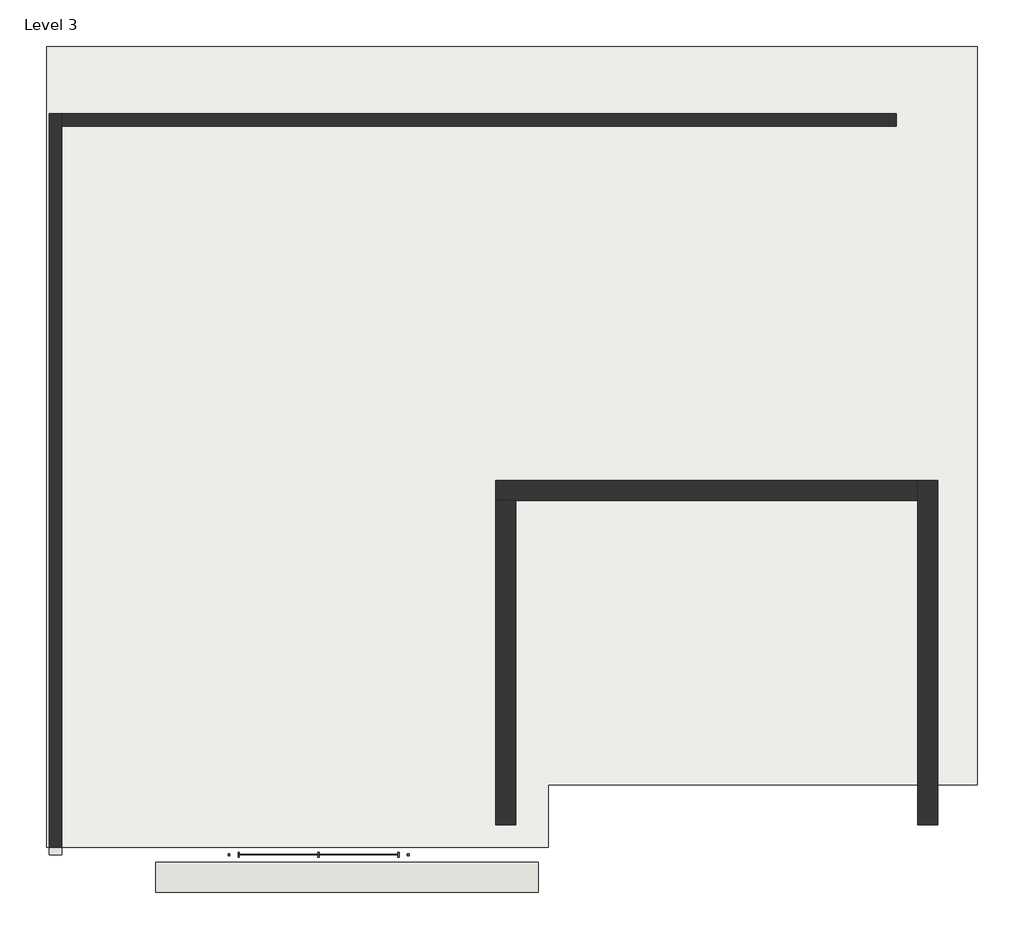
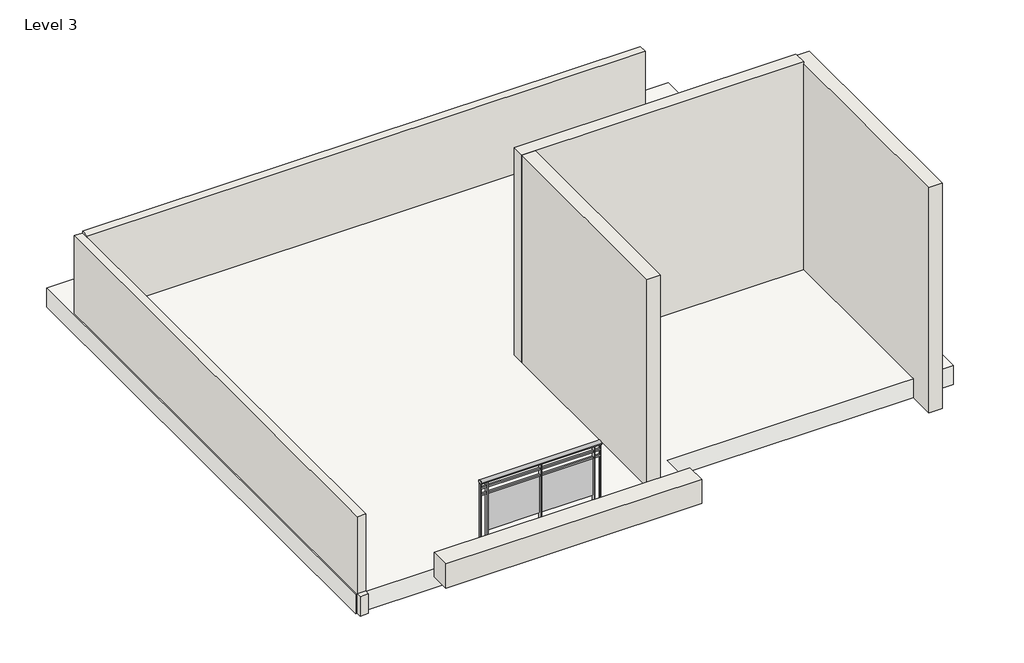
# One storey: 6 walls, 1 railing, 1 roof.
"""IFC4 building model written with IfcOpenShell, lengths in millimetres."""

from ifc_helpers import new_model, si_unit, point, frame, origin, place, context, project, spatial, polyline, ellipse_curve, trimmed, outline, extrude, faceted_brep, transform, mapped, element, save
from ifc_brep_helpers import plane_surface, extruded_surface, advanced_brep
from components import walls_3_walls_3_34f02fba

model = new_model("IFC4")

# Units and contexts
model_context = context("Model", 3, world=origin())
ifc_project = project(units=[si_unit("LENGTHUNIT", "METRE", prefix="MILLI")], contexts=[model_context])

# Site, building, storey
site = spatial("IfcSite", under=ifc_project)
building = spatial("IfcBuilding", under=site)
storey = spatial("IfcBuildingStorey", under=building, Name="Level 3", Elevation=7315.2)

# Railing
placement = place(None, origin())
element("IfcRailing", 1, ObjectType="Glass Panel - Bottom Fill", at=placement, inside=storey, context=model_context, shape_type="SolidModel", body=[
    advanced_brep(
    [(-8387.3093643, 1747.2827135, 8839.2), (-8387.3093643, 1671.0827135, 8839.2), (-6558.5093643, 1747.2827135, 8839.2), (-6558.5093643, 1671.0827135, 8839.2)],
    [
        (0, 1, ellipse_curve(frame((-8387.3093643, 1709.1827135, 8839.2), z_axis=(-1.0, 0.0, 0.0), x_axis=(0.0, -1.0, 0.0)), 38.1, 28.575)),
        (1, 0, ellipse_curve(frame((-8387.3093643, 1709.1827135, 8839.2), z_axis=(-1.0, 0.0, 0.0), x_axis=(0.0, -1.0, 0.0)), 38.1, 28.575)),
        (2, 3, ellipse_curve(frame((-6558.5093643, 1709.1827135, 8839.2), z_axis=(1.0, 0.0, 0.0), x_axis=(0.0, -1.0, 0.0)), 38.1, 28.575)),
        (3, 2, ellipse_curve(frame((-6558.5093643, 1709.1827135, 8839.2), z_axis=(1.0, 0.0, 0.0), x_axis=(0.0, -1.0, 0.0)), 38.1, 28.575)),
        (0, 2),
        (3, 1),
    ],
    [
        plane_surface(frame((-8387.3093643, 1709.1827135, 8839.2), z_axis=(-1.0, 0.0, 0.0), x_axis=(0.0, 1.0, 0.0))),
        plane_surface(frame((-6558.5093643, 1709.1827135, 8839.2), z_axis=(1.0, 0.0, 0.0), x_axis=(0.0, 1.0, 0.0))),
        extruded_surface(trimmed(ellipse_curve(frame((-6558.5093643, 1709.1827135, 8839.2), z_axis=(-1.0, 0.0, 0.0), x_axis=(0.0, -1.0, 0.0)), 38.1, 28.575), [point((-6558.5093643, 1747.2827135, 8839.2))], [point((-6558.5093643, 1671.0827135, 8839.2))], True, "CARTESIAN"), (-1828.7999999999993, 0.0, 0.0), 1828.7999999999993),
        extruded_surface(trimmed(ellipse_curve(frame((-6558.5093643, 1709.1827135, 8839.2), z_axis=(-1.0, 0.0, 0.0), x_axis=(0.0, -1.0, 0.0)), 38.1, 28.575), [point((-6558.5093643, 1671.0827135, 8839.2))], [point((-6558.5093643, 1747.2827135, 8839.2))], True, "CARTESIAN"), (-1828.7999999999993, 0.0, 0.0), 1828.7999999999993),
    ],
    [
        (0, [[1, 2]]),
        (1, [[3, 4]]),
        (2, [[-1, 5, -4, 6]]),
        (3, [[-2, -6, -3, -5]]),
    ],
),
    extrude(outline(polyline([(-8387.3093643, 1696.4827135), (-8387.3093643, 1721.8827135), (-6558.5093643, 1721.8827135), (-6558.5093643, 1696.4827135), (-8387.3093643, 1696.4827135)])), frame((0.0, 0.0, 8724.9), z_axis=(0.0, 0.0, 1.0), x_axis=(1.0, 0.0, 0.0)), (0.0, 0.0, 1.0), 25.4),
    extrude(outline(polyline([(-8387.3093643, 1696.4827135), (-8387.3093643, 1721.8827135), (-6558.5093643, 1721.8827135), (-6558.5093643, 1696.4827135), (-8387.3093643, 1696.4827135)])), frame((0.0, 0.0, 8623.3), z_axis=(0.0, 0.0, 1.0), x_axis=(1.0, 0.0, 0.0)), (0.0, 0.0, 1.0), 25.4),
    extrude(outline(polyline([(-6666.4593643, 1683.7827135), (-6666.4593643, 1734.5827135), (-6653.7593643, 1734.5827135), (-6653.7593643, 1683.7827135), (-6666.4593643, 1683.7827135)])), frame((0.0, 0.0, 7924.8), z_axis=(0.0, 0.0, 1.0), x_axis=(1.0, 0.0, 0.0)), (0.0, 0.0, 1.0), 885.6788223),
    extrude(outline(polyline([(-7472.9093643, 1715.7178705), (-6660.1093643, 1715.7178705), (-6660.1093643, 1709.3678705), (-7472.9093643, 1709.3678705), (-7472.9093643, 1715.7178705)])), frame((0.0, 0.0, 8026.4), z_axis=(0.0, 0.0, 1.0), x_axis=(1.0, 0.0, 0.0)), (0.0, 0.0, 1.0), 596.9),
    extrude(outline(polyline([(-7479.2593643, 1683.7827135), (-7479.2593643, 1734.5827135), (-7466.5593643, 1734.5827135), (-7466.5593643, 1683.7827135), (-7479.2593643, 1683.7827135)])), frame((0.0, 0.0, 7924.8), z_axis=(0.0, 0.0, 1.0), x_axis=(1.0, 0.0, 0.0)), (0.0, 0.0, 1.0), 885.6788223),
    extrude(outline(polyline([(-8285.7093643, 1715.7178705), (-7472.9093643, 1715.7178705), (-7472.9093643, 1709.3678705), (-8285.7093643, 1709.3678705), (-8285.7093643, 1715.7178705)])), frame((0.0, 0.0, 8026.4), z_axis=(0.0, 0.0, 1.0), x_axis=(1.0, 0.0, 0.0)), (0.0, 0.0, 1.0), 596.9),
    extrude(outline(polyline([(-8292.0593643, 1683.7827135), (-8292.0593643, 1734.5827135), (-8279.3593643, 1734.5827135), (-8279.3593643, 1683.7827135), (-8292.0593643, 1683.7827135)])), frame((0.0, 0.0, 7924.8), z_axis=(0.0, 0.0, 1.0), x_axis=(1.0, 0.0, 0.0)), (0.0, 0.0, 1.0), 885.6788223),
    extrude(outline(polyline([(-6571.2093643, 1699.6577135), (-6571.2093643, 1718.7077135), (-6552.1593643, 1718.7077135), (-6552.1593643, 1699.6577135), (-6571.2093643, 1699.6577135)])), frame((0.0, 0.0, 7924.8), z_axis=(0.0, 0.0, 1.0), x_axis=(1.0, 0.0, 0.0)), (0.0, 0.0, 1.0), 885.6788223),
    extrude(outline(polyline([(-8393.6593643, 1699.6577135), (-8393.6593643, 1718.7077135), (-8374.6093643, 1718.7077135), (-8374.6093643, 1699.6577135), (-8393.6593643, 1699.6577135)])), frame((0.0, 0.0, 7924.8), z_axis=(0.0, 0.0, 1.0), x_axis=(1.0, 0.0, 0.0)), (0.0, 0.0, 1.0), 885.6788223),
])

# Roof
element("IfcRoof", 2, ObjectType="Generic - 12\"", at=placement, inside=storey, context=model_context, shape_type="SweptSolid", body=[
    extrude(outline(polyline([(-9504.9093643, 9938.7827135), (-767.3093643, 9938.7827135), (-767.3093643, 2420.3827135), (-5136.1093643, 2420.3827135), (-5136.1093643, 1785.3827135), (-10241.5093643, 1785.3827135), (-10241.5093643, 9938.7827135), (-9504.9093643, 9938.7827135)])), frame((0.0, 0.0, 7315.2), z_axis=(0.0, 0.0, 1.0), x_axis=(1.0, 0.0, 0.0)), (0.0, 0.0, 1.0), 304.8),
])

# Walls
element("IfcWall", 3, ObjectType="Generic - 5\"", at=placement, inside=storey, context=model_context, shape_type="Brep", body=[
    faceted_brep([(-10089.1093643, 1709.1827135, 7315.2), (-10089.1093643, 9125.9827135, 7315.2), (-10089.1093643, 9252.9827135, 7315.2), (-10089.1093643, 9252.9827135, 8872.1089518), (-10089.1093643, 1785.3827135, 8872.1089518), (-10089.1093643, 1785.3827135, 7630.5573397), (-10089.1093643, 1709.1827135, 7630.5573397), (-10216.1093643, 1709.1827135, 7315.2), (-10216.1093643, 1709.1827135, 7630.5573397), (-10216.1093643, 1785.3827135, 7630.5573397), (-10216.1093643, 1785.3827135, 8872.1089518), (-10216.1093643, 9252.9827135, 8872.1089518), (-10216.1093643, 9252.9827135, 7315.2)], [[[0, 1, 2, 3, 4, 5, 6]], [[7, 8, 9, 10, 11, 12]], [[2, 1, 0, 7, 12]], [[4, 3, 11, 10]], [[0, 6, 8, 7]], [[5, 9, 8, 6]], [[5, 4, 10, 9]], [[3, 2, 12, 11]]]),
])
element("IfcWall", 4, ObjectType="Generic - 5\"", at=placement, inside=storey, context=model_context, shape_type="Brep", body=[
    faceted_brep([(-10089.1093643, 9125.9827135, 7315.2), (-1592.8093643, 9125.9827135, 7315.2), (-1592.8093643, 9125.9827135, 8904.3757388), (-10089.1093643, 9125.9827135, 8904.3757388), (-10089.1093643, 9252.9827135, 7315.2), (-10089.1093643, 9252.9827135, 8872.1089518), (-10089.1093643, 9252.9827135, 8904.3757388), (-1592.8093643, 9252.9827135, 8904.3757388), (-1592.8093643, 9252.9827135, 7315.2)], [[[0, 1, 2, 3]], [[4, 5, 6, 7, 8]], [[1, 0, 4, 8]], [[2, 1, 8, 7]], [[3, 2, 7, 6]], [[0, 3, 6, 5, 4]]]),
])
element("IfcWall", 5, ObjectType="Generic - 8\"", at=placement, inside=storey, context=model_context, shape_type="Brep", body=[
    faceted_brep([(-1173.7093643, 2013.9827135, 7315.2), (-1173.7093643, 5519.1827135, 7315.2), (-1173.7093643, 5519.1827135, 10942.7791309), (-1173.7093643, 2013.9827135, 10942.7791309), (-1376.9093643, 2013.9827135, 7315.2), (-1376.9093643, 2013.9827135, 10942.7791309), (-1376.9093643, 5519.1827135, 10942.7791309), (-1376.9093643, 5519.1827135, 7315.2), (-1376.9093643, 5315.9827135, 7315.2)], [[[0, 1, 2, 3]], [[4, 5, 6, 7, 8]], [[1, 0, 4, 8, 7]], [[3, 2, 6, 5]], [[0, 3, 5, 4]], [[2, 1, 7, 6]]]),
])
element("IfcWall", 6, ObjectType="Generic - 8\"", at=placement, inside=storey, context=model_context, shape_type="Brep", body=[
    faceted_brep([(-1376.9093643, 5519.1827135, 7315.2), (-5669.5093643, 5519.1827135, 7315.2), (-5669.5093643, 5519.1827135, 10968.5857686), (-1376.9093643, 5519.1827135, 10968.5857686), (-1376.9093643, 5519.1827135, 10942.7791309), (-1376.9093643, 5315.9827135, 7315.2), (-1376.9093643, 5315.9827135, 10968.5857686), (-5669.5093643, 5315.9827135, 10968.5857686), (-5669.5093643, 5315.9827135, 10967.8023446), (-5669.5093643, 5315.9827135, 7315.2), (-5466.3093643, 5315.9827135, 7315.2)], [[[0, 1, 2, 3, 4]], [[5, 6, 7, 8, 9, 10]], [[1, 0, 5, 10, 9]], [[3, 2, 7, 6]], [[0, 4, 3, 6, 5]], [[2, 1, 9, 8, 7]]]),
])
element("IfcWall", 7, ObjectType="Generic - 8\"", at=placement, inside=storey, context=model_context, shape_type="SweptSolid", body=[
    extrude(outline(polyline([(-5669.5093643, 2013.9827135), (-5669.5093643, 5315.9827135), (-5466.3093643, 5315.9827135), (-5466.3093643, 2013.9827135), (-5669.5093643, 2013.9827135)])), frame((0.0, 0.0, 7315.2), z_axis=(0.0, 0.0, 1.0), x_axis=(1.0, 0.0, 0.0)), (0.0, 0.0, 1.0), 3652.6023446),
])
walls_3_walls_3_shape = walls_3_walls_3_34f02fba(model_context)
element("IfcWall", 8, ObjectType="Walls 3 : Walls 3", at=placement, inside=storey, context=model_context, shape_type="MappedRepresentation", body=[
    mapped(walls_3_walls_3_shape, transform((0.0, 0.0, 0.0), x_axis=(1.0, 0.0, 0.0), y_axis=(0.0, 1.0, 0.0), z_axis=(0.0, 0.0, 1.0))),
])

save(model, "model.ifc")

# Revit data of these elements
# Type "Glass Panel - Bottom Fill"
#   Assembly Code = "C2010400"
#   built-in parameter 1008612 = 0.0416667 (stored number, unit not read)
#   built-in parameter 1008611 = 0.0416667 (stored number, unit not read)
#   built-in parameter 1008609 = 0.333333 (stored number, unit not read)
#   built-in parameter 1008604 = 0.166667 (stored number, unit not read)
#   built-in parameter 1008603 = 0.166667 (stored number, unit not read)
#   Railing Height = 3' - 0"
#   built-in parameter 1008630 = 2
#   built-in parameter 1008610 = 2
#   built-in parameter 1008618 = Baluster - Square : 3/4"
# Type "Generic - 12\""
#   Assembly Code = "B1020"
#   Layers, outside or top first: 1' - 0" no material (function 1)
# Type "Generic - 5\""
#   Assembly Code = "B2010"
#   Layers, outside or top first: 0' - 5" no material (function 1)
# Type "Generic - 8\""
#   Assembly Code = "B2010"
#   Layers, outside or top first: 0' - 8" no material (function 1)
# Element 1 (IfcRailing, "Glass Panel - Bottom Fill")
#   built-in parameter 1008621 = 2 (stored number, unit not read)
#   Phase Created = New Construction
#   Materials on its faces: "Glass"
# Element 2 (IfcRoof, "Generic - 12\"")
#   built-in parameter 1001705 = 25 (stored number, unit not read)
#   built-in parameter 1001710 = 33615
#   Phase Created = New Construction
#   Materials on its faces: "Default Roof"
# Element 3 (IfcWall, "Generic - 5\"")
#   Top Offset = -6' - 10.70437"
#   Base Offset = 0' - 0"
#   wall height = 5' - 1.29563"
#   Phase Created = New Construction
#   Base Constraint = Level 3
#   Top Constraint = Level 4
#   Materials on its faces: "Default Wall"
# Element 4 (IfcWall, "Generic - 5\"")
#   Top Offset = -6' - 9.43403"
#   Base Offset = 0' - 0"
#   wall height = 5' - 2.56597"
#   Phase Created = New Construction
#   Base Constraint = Level 3
#   Top Constraint = Level 4
#   Materials on its faces: "Default Wall"
# Element 5 (IfcWall, "Generic - 8\"")
#   Top Offset = 0' - 0"
#   Base Offset = 0' - 0"
#   Unconnected Height = 11' - 10.81808"
#   wall height = 11' - 10.81808"
#   Phase Created = New Construction
#   Base Constraint = Level 3
#   Materials on its faces: "Default Wall"
# Element 6 (IfcWall, "Generic - 8\"")
#   Top Offset = 0' - 0"
#   Base Offset = 0' - 0"
#   Unconnected Height = 11' - 11.83409"
#   wall height = 11' - 11.83409"
#   Phase Created = New Construction
#   Base Constraint = Level 3
#   Materials on its faces: "Default Wall"
# Element 7 (IfcWall, "Generic - 8\"")
#   Top Offset = 0' - 0"
#   Base Offset = 0' - 0"
#   Unconnected Height = 11' - 11.80324"
#   wall height = 11' - 11.80324"
#   Phase Created = New Construction
#   Base Constraint = Level 3
#   Materials on its faces: "Default Wall"
# Element 8 (IfcWall, "Walls 3 : Walls 3")
#   Phase Created = New Construction
#   Materials on its faces: "Default Wall"
# Materials
#   "Glass": class "Glass", colour RGB 0 128 192, transparency 0.75, Description = "Soda Lime Glass", Cost = 0
#   "Default Roof": colour RGB 88 101 114, transparency 0
#   "Default Wall": colour RGB 128 128 128, transparency 0
